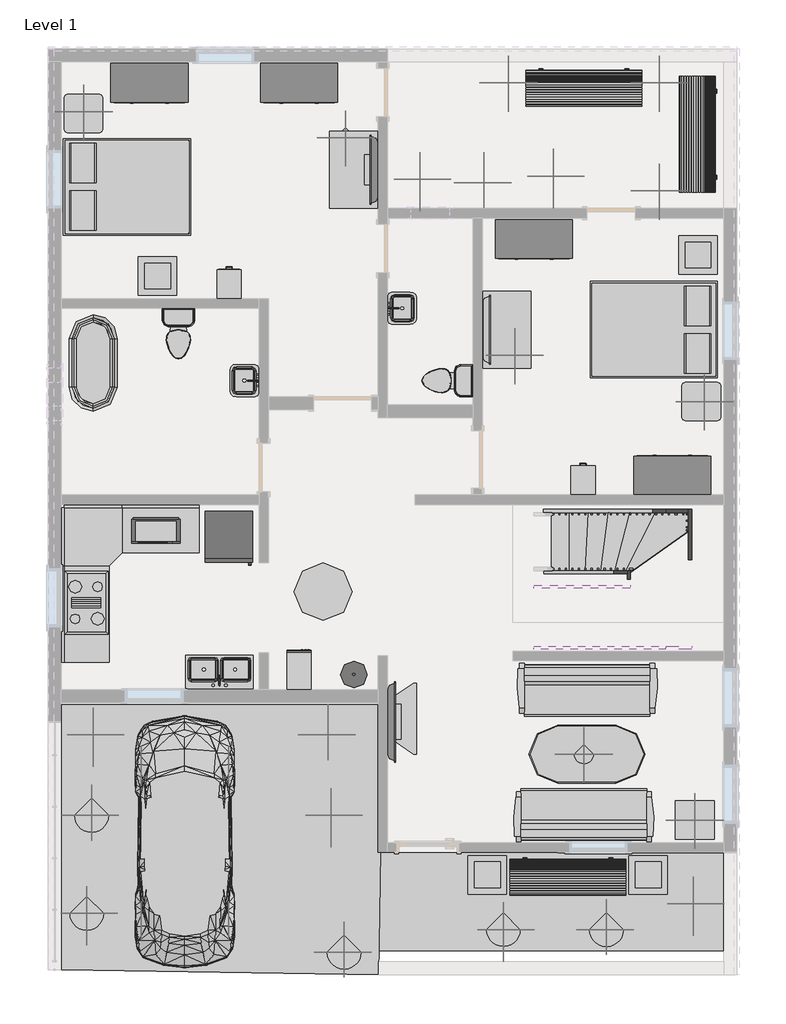
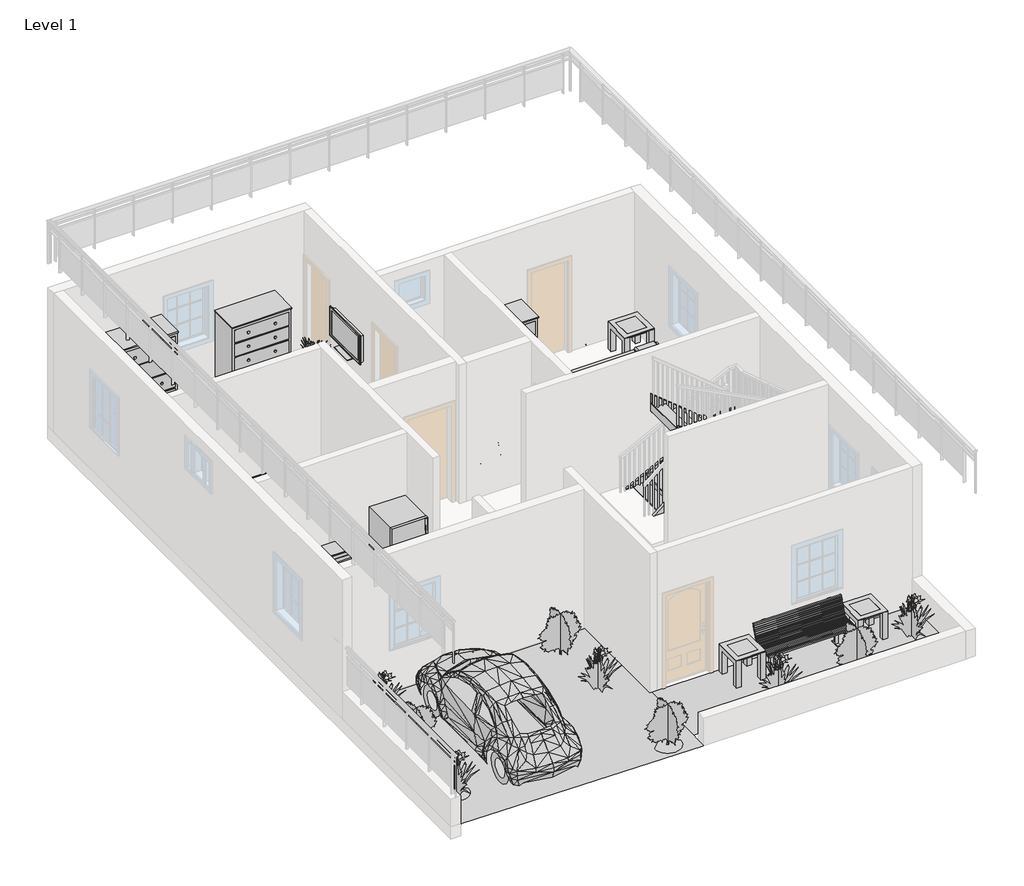
# One storey, part 4 of 4: 26 furniture elements, 24 geographic elements, 9 flow terminals, 8 members, 8 proxies, 1 stair flight.
"""IFC4 building model written with IfcOpenShell, lengths in millimetres."""

from ifc_helpers import new_model, si_unit, frame, origin, place, context, project, spatial, polyline, outline, extrude, triangles, transform, mapped, element, save
from components import proxy_db4bb64d, proxy_bb1e6e30, proxy_8a8d5ab2, rpc_beetle_rpc_beetle_3ce7ba48, proxy_a13a33b2, flow_terminal_2b63360b, flow_terminal_a53be723, flow_terminal_d49f872f, flow_terminal_62a433f7, toilet_domestic_3d_toilet_domestic_3d_f7549cf7, toilet_domestic_3d_toilet_domestic_3d_183bbd19, flow_terminal_b374fae2, furniture_1d2926bd, furniture_bb55ed6b, furniture_2babcf72, furniture_9fa109b2, furniture_aff9b2fb, furniture_7a3aaa4f, furniture_fdf74506, tv_stand_tv_stand_6ce107e5, furniture_b5c51a22, furniture_2c34a4f9, furniture_905aceb5, furniture_31d08a24, furniture_5bc9ed15, furniture_1bba2e14, furniture_3226db35, geographic_element_235d1464, rpc_plant_tropical_55f6ff97, rpc_plant_tropical_agave_1_5_93a2a214, rpc_plant_tropical_jungle_flame_3_9c4808c2, stair_flight_bfa9ce03

model = new_model("IFC4")

# Units and contexts
model_context = context("Model", 3, world=origin())
ifc_project = project(units=[si_unit("LENGTHUNIT", "METRE", prefix="MILLI")], contexts=[model_context])

# Site, building, storey
site = spatial("IfcSite", under=ifc_project)
building = spatial("IfcBuilding", under=site)
storey = spatial("IfcBuildingStorey", under=building, Name="Level 1", Elevation=0.0)

# Proxies
placement = place(None, origin())
element("IfcBuildingElementProxy", 1, Name="Building Element Proxy", at=placement, inside=storey, context=model_context, shape_type="Tessellation", body=[
    triangles([(-7623.7869781, 15698.6789795, 0.0), (-7623.7869781, 13031.6789795, 0.0), (-2111.986639, 15698.6789795, 0.0), (-2111.986639, 13184.0789795, 0.0)], [[1, 2, 4], [4, 3, 1]], closed=False),
])
element("IfcBuildingElementProxy", 2, Name="Building Element Proxy", at=placement, inside=storey, context=model_context, shape_type="Tessellation", body=[
    triangles([(-12983.1865906, 5475.1785919, 0.0), (-7699.9869781, 5487.8789795, 0.0), (-7763.4865906, 1474.6787373, 0.0), (-12983.1865906, 1576.2787857, 0.0), (-12779.986203, 1169.8788099, 0.0), (-7763.4865906, 1093.6788099, 0.0)], [[2, 1, 4], [3, 4, 5], [3, 6, 2], [6, 3, 5], [3, 2, 4]], closed=False),
])
element("IfcBuildingElementProxy", 3, Name="Building Element Proxy", at=placement, inside=storey, context=model_context, shape_type="Tessellation", body=[
    triangles([(-7776.1869781, 3024.0787857, 0.0), (-7763.4865906, 1474.6787373, 0.0), (-2111.986639, 3011.3786888, 0.0), (-2111.986639, 1474.6787373, 0.0)], [[1, 2, 3], [4, 3, 2]], closed=False),
])
proxy_shape = proxy_db4bb64d(model_context)
element("IfcBuildingElementProxy", 4, Name="15\" x 24\" x 34 1/2\"", ObjectType="15\" x 24\" x 34 1/2\"", at=placement, inside=storey, context=model_context, shape_type="MappedRepresentation", body=[
    mapped(proxy_shape, transform((-8752.769227, 6160.7283581, 0.0), x_axis=(-0.9999999999999998, 0.0, 0.0), y_axis=(0.0, -0.9999999999999998, 0.0), z_axis=(0.0, 0.0, 1.0))),
])
proxy_2_shape = proxy_bb1e6e30(model_context)
element("IfcBuildingElementProxy", 5, Name="Cook Top-4 Unit : 36\" x 20\"", ObjectType="Cook Top-4 Unit : 36\" x 20\"", at=placement, inside=storey, context=model_context, shape_type="MappedRepresentation", body=[
    mapped(proxy_2_shape, transform((-12379.9366955, 6961.0787933, 0.0), x_axis=(0.0, 1.0000000000000002, 0.0), y_axis=(-1.0000000000000002, 0.0, 0.0), z_axis=(0.0, 0.0, 1.0))),
])
proxy_3_shape = proxy_8a8d5ab2(model_context)
element("IfcBuildingElementProxy", 6, Name="Microwave : 30\" x 16\" x 18\"", ObjectType="Microwave : 30\" x 16\" x 18\"", at=placement, inside=storey, context=model_context, shape_type="MappedRepresentation", body=[
    mapped(proxy_3_shape, transform((-11781.6795729, 8457.1592991, 0.0), x_axis=(1.0000000000000009, 0.0, 0.0), y_axis=(0.0, 1.0000000000000009, 0.0), z_axis=(0.0, 0.0, 1.0))),
])
rpc_beetle_rpc_beetle_shape = rpc_beetle_rpc_beetle_3ce7ba48(model_context)
element("IfcBuildingElementProxy", 7, Name="RPC Beetle : RPC Beetle", ObjectType="RPC Beetle : RPC Beetle", at=placement, inside=storey, context=model_context, shape_type="MappedRepresentation", body=[
    mapped(rpc_beetle_rpc_beetle_shape, transform((-10824.1866955, 1957.2787933, 0.0), x_axis=(1.0, 0.0, 0.0), y_axis=(0.0, 1.0, 0.0), z_axis=(0.0, 0.0, 1.0))),
])
proxy_4_shape = proxy_a13a33b2(model_context)
element("IfcBuildingElementProxy", 8, Name="Refrigerator : 30\" x 32\" RH", ObjectType="Refrigerator : 30\" x 32\" RH", at=placement, inside=storey, context=model_context, shape_type="MappedRepresentation", body=[
    mapped(proxy_4_shape, transform((-10130.4491955, 8020.3298218, 0.0), x_axis=(1.0, 0.0, 0.0), y_axis=(0.0, 1.0, 0.0), z_axis=(0.0, 0.0, 1.0))),
])

# Flow terminals
flow_terminal_shape = flow_terminal_2b63360b(model_context)
element("IfcFlowTerminal", 9, ObjectType="Floor Drain - Rectangular : 5\"x5\" Strainer - 2\" Drain", at=placement, inside=storey, context=model_context, shape_type="MappedRepresentation", body=[
    mapped(flow_terminal_shape, transform((-11687.7866955, 11152.0787933, 0.0), x_axis=(1.0, 0.0, 0.0), y_axis=(0.0, 1.0, 0.0), z_axis=(0.0, 0.0, 1.0))),
])
element("IfcFlowTerminal", 10, ObjectType="Floor Drain - Rectangular : 5\"x5\" Strainer - 2\" Drain", at=placement, inside=storey, context=model_context, shape_type="MappedRepresentation", body=[
    mapped(flow_terminal_shape, transform((-7420.5866955, 10694.8787933, 0.0), x_axis=(1.0, 0.0, 0.0), y_axis=(0.0, 1.0, 0.0), z_axis=(0.0, 0.0, 1.0))),
])
flow_terminal_2_shape = flow_terminal_a53be723(model_context)
element("IfcFlowTerminal", 11, ObjectType="Sink Kitchen-Double : 42\" x 21\"", at=placement, inside=storey, context=model_context, shape_type="MappedRepresentation", body=[
    mapped(flow_terminal_2_shape, transform((-10262.397455, 5871.2241944, 0.0), x_axis=(-1.0000000000000004, 0.0, 0.0), y_axis=(0.0, -1.0000000000000004, 0.0), z_axis=(0.0, 0.0, 1.0))),
])
flow_terminal_3_shape = flow_terminal_d49f872f(model_context)
element("IfcFlowTerminal", 12, ObjectType="Sink Vanity-Round : 19\" x 19\"", at=placement, inside=storey, context=model_context, shape_type="MappedRepresentation", body=[
    mapped(flow_terminal_3_shape, transform((-8060.534955, 5914.6658677, 609.6), x_axis=(-1.0000000000000004, 0.0, 0.0), y_axis=(0.0, -1.0000000000000004, 0.0), z_axis=(0.0, 0.0, 1.0))),
])
flow_terminal_4_shape = flow_terminal_62a433f7(model_context)
element("IfcFlowTerminal", 13, ObjectType="Sink Vanity-Square : 20\" x 18\"", at=placement, inside=storey, context=model_context, shape_type="MappedRepresentation", body=[
    mapped(flow_terminal_4_shape, transform((-9835.9320966, 10481.9680338, 0.0), x_axis=(0.0, -0.9999999999999999, 0.0), y_axis=(0.9999999999999999, 0.0, 0.0), z_axis=(0.0, 0.0, 1.0))),
])
element("IfcFlowTerminal", 14, ObjectType="Sink Vanity-Square : 20\" x 18\"", at=placement, inside=storey, context=model_context, shape_type="MappedRepresentation", body=[
    mapped(flow_terminal_4_shape, transform((-7443.6412944, 11593.5895527, 0.0), x_axis=(0.0, 1.0000000000000002, 0.0), y_axis=(-1.0000000000000002, 0.0, 0.0), z_axis=(0.0, 0.0, 1.0))),
])
toilet_domestic_3d_toilet_domestic_3d_shape = toilet_domestic_3d_toilet_domestic_3d_f7549cf7(model_context)
toilet_domestic_3d_toilet_domestic_3d_2_shape = toilet_domestic_3d_toilet_domestic_3d_183bbd19(model_context)
element("IfcFlowTerminal", 15, ObjectType="Toilet-Domestic-3D : Toilet-Domestic-3D", at=placement, inside=storey, context=model_context, shape_type="MappedRepresentation", body=[
    mapped(toilet_domestic_3d_toilet_domestic_3d_shape, transform((-10925.7866955, 11114.5827659, 0.0), x_axis=(1.0, 0.0, 0.0), y_axis=(0.0, 1.0, 0.0), z_axis=(0.0, 0.0, 1.0))),
    mapped(toilet_domestic_3d_toilet_domestic_3d_2_shape, transform((-10925.7866955, 11114.5827659, 0.0), x_axis=(1.0, 0.0, 0.0), y_axis=(0.0, 1.0, 0.0), z_axis=(0.0, 0.0, 1.0))),
])
element("IfcFlowTerminal", 16, ObjectType="Toilet-Domestic-3D : Toilet-Domestic-3D", at=placement, inside=storey, context=model_context, shape_type="MappedRepresentation", body=[
    mapped(toilet_domestic_3d_toilet_domestic_3d_shape, transform((-6772.2827229, 10466.2787933, 0.0), x_axis=(0.0, -1.0, 0.0), y_axis=(1.0, 0.0, 0.0), z_axis=(0.0, 0.0, 1.0))),
    mapped(toilet_domestic_3d_toilet_domestic_3d_2_shape, transform((-6772.2827229, 10466.2787933, 0.0), x_axis=(0.0, -1.0, 0.0), y_axis=(1.0, 0.0, 0.0), z_axis=(0.0, 0.0, 1.0))),
])
flow_terminal_5_shape = flow_terminal_b374fae2(model_context)
element("IfcFlowTerminal", 17, ObjectType="Tub-Free Standing-3D : 30\" x 60\"", at=placement, inside=storey, context=model_context, shape_type="MappedRepresentation", body=[
    mapped(flow_terminal_5_shape, transform((-12271.9866955, 10745.6787933, 0.0), x_axis=(1.0, 0.0, 0.0), y_axis=(0.0, 1.0, 0.0), z_axis=(0.0, 0.0, 1.0))),
])

# Furniture
furniture_shape = furniture_1d2926bd(model_context)
element("IfcFurniture", 18, ObjectType="Bed-Box : Queen 60\" x 79\"", at=placement, inside=storey, context=model_context, shape_type="MappedRepresentation", body=[
    mapped(furniture_shape, transform((-11973.0162037, 13184.0787933, 0.0), x_axis=(0.0, 1.0000000000000002, 0.0), y_axis=(-1.0000000000000002, 0.0, 0.0), z_axis=(0.0, 0.0, 1.0))),
])
element("IfcFurniture", 19, ObjectType="Bed-Box : Queen 60\" x 79\"", at=placement, inside=storey, context=model_context, shape_type="MappedRepresentation", body=[
    mapped(furniture_shape, transform((-3185.6571873, 11609.2787933, 0.0), x_axis=(0.0, -1.0000000000000009, 0.0), y_axis=(1.0000000000000009, 0.0, 0.0), z_axis=(0.0, 0.0, 1.0))),
])
furniture_2_shape = furniture_bb55ed6b(model_context)
element("IfcFurniture", 20, ObjectType="Cabinet-File 2 Drawer : 15\" x 18\"", at=placement, inside=storey, context=model_context, shape_type="MappedRepresentation", body=[
    mapped(furniture_2_shape, transform((-10253.5831426, 11848.1444931, 0.0), x_axis=(-1.0000000000000002, 0.0, 0.0), y_axis=(0.0, -1.0000000000000002, 0.0), z_axis=(0.0, 0.0, 1.0))),
])
element("IfcFurniture", 21, ObjectType="Cabinet-File 2 Drawer : 15\" x 18\"", at=placement, inside=storey, context=model_context, shape_type="MappedRepresentation", body=[
    mapped(furniture_2_shape, transform((-4665.5831426, 8749.3444931, 0.0), x_axis=(-1.0, 0.0, 0.0), y_axis=(0.0, -1.0, 0.0), z_axis=(0.0, 0.0, 1.0))),
])
furniture_3_shape = furniture_2babcf72(model_context)
element("IfcFurniture", 22, ObjectType="Dresser : 48\" x 60\" x 24\"", at=placement, inside=storey, context=model_context, shape_type="MappedRepresentation", body=[
    mapped(furniture_3_shape, transform((-8751.5934357, 15528.4417474, 0.0), x_axis=(1.0, 0.0, 0.0), y_axis=(0.0, 1.0, 0.0), z_axis=(0.0, 0.0, 1.0))),
])
element("IfcFurniture", 23, ObjectType="Dresser : 48\" x 60\" x 24\"", at=placement, inside=storey, context=model_context, shape_type="MappedRepresentation", body=[
    mapped(furniture_3_shape, transform((-5043.1934357, 13064.6417474, 0.0), x_axis=(1.0, 0.0, 0.0), y_axis=(0.0, 1.0, 0.0), z_axis=(0.0, 0.0, 1.0))),
])
furniture_4_shape = furniture_9fa109b2(model_context)
element("IfcFurniture", 24, ObjectType="Dresser : 48\" x 72\" x 24\"", at=placement, inside=storey, context=model_context, shape_type="MappedRepresentation", body=[
    mapped(furniture_4_shape, transform((-11113.7934357, 15528.4417474, 0.0), x_axis=(1.0, 0.0, 0.0), y_axis=(0.0, 1.0, 0.0), z_axis=(0.0, 0.0, 1.0))),
])
element("IfcFurniture", 25, ObjectType="Dresser : 48\" x 72\" x 24\"", at=placement, inside=storey, context=model_context, shape_type="MappedRepresentation", body=[
    mapped(furniture_4_shape, transform((-3397.1799554, 8604.5158392, 0.0), x_axis=(-1.000000000000001, 0.0, 0.0), y_axis=(0.0, -1.000000000000001, 0.0), z_axis=(0.0, 0.0, 1.0))),
])
furniture_5_shape = furniture_aff9b2fb(model_context)
element("IfcFurniture", 26, ObjectType="Sofa-Pensi : 84\"", at=placement, inside=storey, context=model_context, shape_type="MappedRepresentation", body=[
    mapped(furniture_5_shape, transform((-4246.3804455, 3885.3886293, 0.0), x_axis=(-1.0000000000000004, 0.0, 0.0), y_axis=(0.0, -1.0000000000000004, 0.0), z_axis=(0.0, 0.0, 1.0))),
])
element("IfcFurniture", 27, ObjectType="Sofa-Pensi : 84\"", at=placement, inside=storey, context=model_context, shape_type="MappedRepresentation", body=[
    mapped(furniture_5_shape, transform((-4752.7929455, 5312.3689572, 0.0), x_axis=(1.0000000000000002, 0.0, 0.0), y_axis=(0.0, 1.0000000000000002, 0.0), z_axis=(0.0, 0.0, 1.0))),
])
furniture_6_shape = furniture_7a3aaa4f(model_context)
element("IfcFurniture", 28, ObjectType="TV - Flat Screen : 42\"", at=placement, inside=storey, context=model_context, shape_type="MappedRepresentation", body=[
    mapped(furniture_6_shape, transform((-7834.7253192, 13789.7342791, 990.6), x_axis=(0.0, -1.0000000000000004, 0.0), y_axis=(1.0000000000000004, 0.0, 0.0), z_axis=(0.0, 0.0, 1.0))),
])
element("IfcFurniture", 29, ObjectType="TV - Flat Screen : 42\"", at=placement, inside=storey, context=model_context, shape_type="MappedRepresentation", body=[
    mapped(furniture_6_shape, transform((-6066.6480719, 11274.0708484, 0.0), x_axis=(0.0, 1.0000000000000002, 0.0), y_axis=(-1.0000000000000002, 0.0, 0.0), z_axis=(0.0, 0.0, 1.0))),
])
furniture_7_shape = furniture_fdf74506(model_context)
element("IfcFurniture", 30, ObjectType="TV - Flat Screen : 50\"", at=placement, inside=storey, context=model_context, shape_type="MappedRepresentation", body=[
    mapped(furniture_7_shape, transform((-7565.2480719, 5085.4233074, 914.4), x_axis=(0.0, 1.0000000000000002, 0.0), y_axis=(-1.0000000000000002, 0.0, 0.0), z_axis=(0.0, 0.0, 1.0))),
])
tv_stand_tv_stand_shape = tv_stand_tv_stand_6ce107e5(model_context)
element("IfcFurniture", 31, ObjectType="TV Stand : TV Stand", at=placement, inside=storey, context=model_context, shape_type="MappedRepresentation", body=[
    mapped(tv_stand_tv_stand_shape, transform((-7623.7866955, 5007.0907912, 0.0), x_axis=(0.0, 1.0000000000000002, 0.0), y_axis=(-1.0000000000000002, 0.0, 0.0), z_axis=(0.0, 0.0, 1.0))),
])
furniture_8_shape = furniture_b5c51a22(model_context)
element("IfcFurniture", 32, ObjectType="Table-Coffee : 24\" x 24\" x 24\"", at=placement, inside=storey, context=model_context, shape_type="MappedRepresentation", body=[
    mapped(furniture_8_shape, transform((-11274.2524622, 12022.0677155, 0.0), x_axis=(1.0, 0.0, 0.0), y_axis=(0.0, 1.0, 0.0), z_axis=(0.0, 0.0, 1.0))),
])
element("IfcFurniture", 33, ObjectType="Table-Coffee : 24\" x 24\" x 24\"", at=placement, inside=storey, context=model_context, shape_type="MappedRepresentation", body=[
    mapped(furniture_8_shape, transform((-2739.8524622, 12352.2677155, 0.0), x_axis=(1.0, 0.0, 0.0), y_axis=(0.0, 1.0, 0.0), z_axis=(0.0, 0.0, 1.0))),
])
element("IfcFurniture", 34, ObjectType="Table-Coffee : 24\" x 24\" x 24\"", at=placement, inside=storey, context=model_context, shape_type="MappedRepresentation", body=[
    mapped(furniture_8_shape, transform((-6067.2524622, 2573.2677155, 0.0), x_axis=(1.0, 0.0, 0.0), y_axis=(0.0, 1.0, 0.0), z_axis=(0.0, 0.0, 1.0))),
])
element("IfcFurniture", 35, ObjectType="Table-Coffee : 24\" x 24\" x 24\"", at=placement, inside=storey, context=model_context, shape_type="MappedRepresentation", body=[
    mapped(furniture_8_shape, transform((-3527.2524622, 2573.2677155, 0.0), x_axis=(1.0, 0.0, 0.0), y_axis=(0.0, 1.0, 0.0), z_axis=(0.0, 0.0, 1.0))),
])
furniture_9_shape = furniture_2c34a4f9(model_context)
element("IfcFurniture", 36, ObjectType="Table-Dining Oval : 36\" x 72\"", at=placement, inside=storey, context=model_context, shape_type="MappedRepresentation", body=[
    mapped(furniture_9_shape, transform((-4072.3670234, 4931.5771539, 0.0), x_axis=(1.0, 0.0, 0.0), y_axis=(0.0, 1.0, 0.0), z_axis=(0.0, 0.0, 1.0))),
])
furniture_10_shape = furniture_905aceb5(model_context)
element("IfcFurniture", 37, ObjectType="Table-Dining Round w Chairs : 36\" Diameter", at=placement, inside=storey, context=model_context, shape_type="MappedRepresentation", body=[
    mapped(furniture_10_shape, transform((-8743.4686627, 7323.7574818, 0.0), x_axis=(1.0, 0.0, 0.0), y_axis=(0.0, 1.0, 0.0), z_axis=(0.0, 0.0, 1.0))),
])
furniture_11_shape = furniture_31d08a24(model_context)
element("IfcFurniture", 38, ObjectType="Table-End : 24\" x 24\"", at=placement, inside=storey, context=model_context, shape_type="MappedRepresentation", body=[
    mapped(furniture_11_shape, transform((-12732.9203258, 14530.2787933, 0.0), x_axis=(1.0, 0.0, 0.0), y_axis=(0.0, 1.0, 0.0), z_axis=(0.0, 0.0, 1.0))),
])
element("IfcFurniture", 39, ObjectType="Table-End : 24\" x 24\"", at=placement, inside=storey, context=model_context, shape_type="MappedRepresentation", body=[
    mapped(furniture_11_shape, transform((-2979.3203258, 9983.6787933, 0.0), x_axis=(1.0, 0.0, 0.0), y_axis=(0.0, 1.0, 0.0), z_axis=(0.0, 0.0, 1.0))),
])
furniture_12_shape = furniture_5bc9ed15(model_context)
element("IfcFurniture", 40, ObjectType="Table-Night Stand : 24\" x 24\" x 30\"", at=placement, inside=storey, context=model_context, shape_type="MappedRepresentation", body=[
    mapped(furniture_12_shape, transform((-2463.8530652, 3836.8787933, 0.0), x_axis=(-1.0000000000000004, 0.0, 0.0), y_axis=(0.0, -1.0000000000000004, 0.0), z_axis=(0.0, 0.0, 1.0))),
])
furniture_13_shape = furniture_1bba2e14(model_context)
element("IfcFurniture", 41, ObjectType="Table-Rectangular : 72\" x 30\"", at=placement, inside=storey, context=model_context, shape_type="MappedRepresentation", body=[
    mapped(furniture_13_shape, transform((-8157.1866955, 13793.6787933, 0.0), x_axis=(0.0, 1.0000000000000002, 0.0), y_axis=(-1.0000000000000002, 0.0, 0.0), z_axis=(0.0, 0.0, 1.0))),
])
element("IfcFurniture", 42, ObjectType="Table-Rectangular : 72\" x 30\"", at=placement, inside=storey, context=model_context, shape_type="MappedRepresentation", body=[
    mapped(furniture_13_shape, transform((-5744.1866955, 11270.1263343, 0.0), x_axis=(0.0, 1.0000000000000002, 0.0), y_axis=(-1.0000000000000002, 0.0, 0.0), z_axis=(0.0, 0.0, 1.0))),
])
furniture_14_shape = furniture_3226db35(model_context)
element("IfcFurniture", 43, ObjectType="Work Station Cubicle : 96\" x 96\"", at=placement, inside=storey, context=model_context, shape_type="MappedRepresentation", body=[
    mapped(furniture_14_shape, transform((-12648.2549433, 9005.5018009, 0.0), x_axis=(1.0, 0.0, 0.0), y_axis=(0.0, 1.0, 0.0), z_axis=(0.0, 0.0, 1.0))),
])

# Geographic elements
geographic_element_shape = geographic_element_235d1464(model_context)
element("IfcGeographicElement", 44, ObjectType="Park Bench : 72\"", at=placement, inside=storey, context=model_context, shape_type="MappedRepresentation", body=[
    mapped(geographic_element_shape, transform((-4524.9866955, 15114.4787933, 0.0), x_axis=(1.0, 0.0, 0.0), y_axis=(0.0, 1.0, 0.0), z_axis=(0.0, 0.0, 1.0))),
])
element("IfcGeographicElement", 45, ObjectType="Park Bench : 72\"", at=placement, inside=storey, context=model_context, shape_type="MappedRepresentation", body=[
    mapped(geographic_element_shape, transform((-2696.1866955, 14352.4787933, 0.0), x_axis=(0.0, -1.0000000000000004, 0.0), y_axis=(1.0000000000000004, 0.0, 0.0), z_axis=(0.0, 0.0, 1.0))),
])
element("IfcGeographicElement", 46, ObjectType="Park Bench : 72\"", at=placement, inside=storey, context=model_context, shape_type="MappedRepresentation", body=[
    mapped(geographic_element_shape, transform((-4778.9866955, 2668.4787933, 0.0), x_axis=(1.0, 0.0, 0.0), y_axis=(0.0, 1.0, 0.0), z_axis=(0.0, 0.0, 1.0))),
])
rpc_plant_tropical_shape = rpc_plant_tropical_55f6ff97(model_context)
element("IfcGeographicElement", 47, ObjectType="RPC Plant - Tropical", at=placement, inside=storey, context=model_context, shape_type="MappedRepresentation", body=[
    mapped(rpc_plant_tropical_shape, transform((-7115.7866955, 13641.2787933, 0.0), x_axis=(1.0, 0.0, 0.0), y_axis=(0.0, 1.0, 0.0), z_axis=(0.0, 0.0, 1.0))),
])
element("IfcGeographicElement", 48, ObjectType="RPC Plant - Tropical", at=placement, inside=storey, context=model_context, shape_type="MappedRepresentation", body=[
    mapped(rpc_plant_tropical_shape, transform((-5007.5866955, 13692.0787933, 0.0), x_axis=(1.0, 0.0, 0.0), y_axis=(0.0, 1.0, 0.0), z_axis=(0.0, 0.0, 1.0))),
])
element("IfcGeographicElement", 49, ObjectType="RPC Plant - Tropical", at=placement, inside=storey, context=model_context, shape_type="MappedRepresentation", body=[
    mapped(rpc_plant_tropical_shape, transform((-12271.9866955, 4878.2787933, 0.0), x_axis=(1.0, 0.0, 0.0), y_axis=(0.0, 1.0, 0.0), z_axis=(0.0, 0.0, 1.0))),
])
element("IfcGeographicElement", 50, ObjectType="RPC Plant - Tropical", at=placement, inside=storey, context=model_context, shape_type="MappedRepresentation", body=[
    mapped(rpc_plant_tropical_shape, transform((-12373.5866955, 2058.8787933, 0.0), x_axis=(1.0, 0.0, 0.0), y_axis=(0.0, 1.0, 0.0), z_axis=(0.0, 0.0, 1.0))),
])
element("IfcGeographicElement", 51, ObjectType="RPC Plant - Tropical", at=placement, inside=storey, context=model_context, shape_type="MappedRepresentation", body=[
    mapped(rpc_plant_tropical_shape, transform((-8512.7866955, 3608.2787933, 0.0), x_axis=(1.0, 0.0, 0.0), y_axis=(0.0, 1.0, 0.0), z_axis=(0.0, 0.0, 1.0))),
])
element("IfcGeographicElement", 52, ObjectType="RPC Plant - Tropical", at=placement, inside=storey, context=model_context, shape_type="MappedRepresentation", body=[
    mapped(rpc_plant_tropical_shape, transform((-2797.7866955, 2211.2787933, 0.0), x_axis=(1.0, 0.0, 0.0), y_axis=(0.0, 1.0, 0.0), z_axis=(0.0, 0.0, 1.0))),
])
element("IfcGeographicElement", 53, ObjectType="RPC Plant - Tropical", at=placement, inside=storey, context=model_context, shape_type="MappedRepresentation", body=[
    mapped(rpc_plant_tropical_shape, transform((-5794.9866955, 1804.8787933, 0.0), x_axis=(1.0, 0.0, 0.0), y_axis=(0.0, 1.0, 0.0), z_axis=(0.0, 0.0, 1.0))),
])
rpc_plant_tropical_agave_1_5_shape = rpc_plant_tropical_agave_1_5_93a2a214(model_context)
element("IfcGeographicElement", 54, ObjectType="RPC Plant - Tropical : Agave - 1.5'", at=placement, inside=storey, context=model_context, shape_type="MappedRepresentation", body=[
    mapped(rpc_plant_tropical_agave_1_5_shape, transform((-12424.3866955, 14708.0787933, 609.6), x_axis=(1.0, 0.0, 0.0), y_axis=(0.0, 1.0, 0.0), z_axis=(0.0, 0.0, 1.0))),
])
element("IfcGeographicElement", 55, ObjectType="RPC Plant - Tropical : Agave - 1.5'", at=placement, inside=storey, context=model_context, shape_type="MappedRepresentation", body=[
    mapped(rpc_plant_tropical_agave_1_5_shape, transform((-8284.1866955, 14301.6787933, 609.6), x_axis=(1.0, 0.0, 0.0), y_axis=(0.0, 1.0, 0.0), z_axis=(0.0, 0.0, 1.0))),
])
element("IfcGeographicElement", 56, ObjectType="RPC Plant - Tropical : Agave - 1.5'", at=placement, inside=storey, context=model_context, shape_type="MappedRepresentation", body=[
    mapped(rpc_plant_tropical_agave_1_5_shape, transform((-3331.1866955, 15165.2787933, 0.0), x_axis=(1.0, 0.0, 0.0), y_axis=(0.0, 1.0, 0.0), z_axis=(0.0, 0.0, 1.0))),
])
element("IfcGeographicElement", 57, ObjectType="RPC Plant - Tropical : Agave - 1.5'", at=placement, inside=storey, context=model_context, shape_type="MappedRepresentation", body=[
    mapped(rpc_plant_tropical_agave_1_5_shape, transform((-5718.7866955, 15165.2787933, 0.0), x_axis=(1.0, 0.0, 0.0), y_axis=(0.0, 1.0, 0.0), z_axis=(0.0, 0.0, 1.0))),
])
element("IfcGeographicElement", 58, ObjectType="RPC Plant - Tropical : Agave - 1.5'", at=placement, inside=storey, context=model_context, shape_type="MappedRepresentation", body=[
    mapped(rpc_plant_tropical_agave_1_5_shape, transform((-3331.1866955, 13463.4787933, 0.0), x_axis=(1.0, 0.0, 0.0), y_axis=(0.0, 1.0, 0.0), z_axis=(0.0, 0.0, 1.0))),
])
element("IfcGeographicElement", 59, ObjectType="RPC Plant - Tropical : Agave - 1.5'", at=placement, inside=storey, context=model_context, shape_type="MappedRepresentation", body=[
    mapped(rpc_plant_tropical_agave_1_5_shape, transform((-2619.9866955, 10136.0787933, 609.6), x_axis=(1.0, 0.0, 0.0), y_axis=(0.0, 1.0, 0.0), z_axis=(0.0, 0.0, 1.0))),
])
element("IfcGeographicElement", 60, ObjectType="RPC Plant - Tropical : Agave - 1.5'", at=placement, inside=storey, context=model_context, shape_type="MappedRepresentation", body=[
    mapped(rpc_plant_tropical_agave_1_5_shape, transform((-5617.1866955, 10863.7263343, 609.6), x_axis=(1.0, 0.0, 0.0), y_axis=(0.0, 1.0, 0.0), z_axis=(0.0, 0.0, 1.0))),
])
element("IfcGeographicElement", 61, ObjectType="RPC Plant - Tropical : Agave - 1.5'", at=placement, inside=storey, context=model_context, shape_type="MappedRepresentation", body=[
    mapped(rpc_plant_tropical_agave_1_5_shape, transform((-4524.9866955, 4573.4787933, 914.4), x_axis=(1.0, 0.0, 0.0), y_axis=(0.0, 1.0, 0.0), z_axis=(0.0, 0.0, 1.0))),
])
element("IfcGeographicElement", 62, ObjectType="RPC Plant - Tropical : Agave - 1.5'", at=placement, inside=storey, context=model_context, shape_type="MappedRepresentation", body=[
    mapped(rpc_plant_tropical_agave_1_5_shape, transform((-2772.3866955, 3532.0787933, 762.0), x_axis=(1.0, 0.0, 0.0), y_axis=(0.0, 1.0, 0.0), z_axis=(0.0, 0.0, 1.0))),
])
rpc_plant_tropical_jungle_flame_3_shape = rpc_plant_tropical_jungle_flame_3_9c4808c2(model_context)
element("IfcGeographicElement", 63, ObjectType="RPC Plant - Tropical : Jungle Flame - 3'", at=placement, inside=storey, context=model_context, shape_type="MappedRepresentation", body=[
    mapped(rpc_plant_tropical_jungle_flame_3_shape, transform((-6099.7866955, 13590.4787933, 0.0), x_axis=(1.0, 0.0, 0.0), y_axis=(0.0, 1.0, 0.0), z_axis=(0.0, 0.0, 1.0))),
])
element("IfcGeographicElement", 64, ObjectType="RPC Plant - Tropical : Jungle Flame - 3'", at=placement, inside=storey, context=model_context, shape_type="MappedRepresentation", body=[
    mapped(rpc_plant_tropical_jungle_flame_3_shape, transform((-12297.3866955, 3608.2787933, 0.0), x_axis=(1.0, 0.0, 0.0), y_axis=(0.0, 1.0, 0.0), z_axis=(0.0, 0.0, 1.0))),
])
element("IfcGeographicElement", 65, ObjectType="RPC Plant - Tropical : Jungle Flame - 3'", at=placement, inside=storey, context=model_context, shape_type="MappedRepresentation", body=[
    mapped(rpc_plant_tropical_jungle_flame_3_shape, transform((-8563.5866955, 4878.2787933, 0.0), x_axis=(1.0, 0.0, 0.0), y_axis=(0.0, 1.0, 0.0), z_axis=(0.0, 0.0, 1.0))),
])
element("IfcGeographicElement", 66, ObjectType="RPC Plant - Tropical : Jungle Flame - 3'", at=placement, inside=storey, context=model_context, shape_type="MappedRepresentation", body=[
    mapped(rpc_plant_tropical_jungle_flame_3_shape, transform((-8309.5866955, 1449.2787933, 0.0), x_axis=(1.0, 0.0, 0.0), y_axis=(0.0, 1.0, 0.0), z_axis=(0.0, 0.0, 1.0))),
])
element("IfcGeographicElement", 67, ObjectType="RPC Plant - Tropical : Jungle Flame - 3'", at=placement, inside=storey, context=model_context, shape_type="MappedRepresentation", body=[
    mapped(rpc_plant_tropical_jungle_flame_3_shape, transform((-4169.3866955, 1804.8787933, 0.0), x_axis=(1.0, 0.0, 0.0), y_axis=(0.0, 1.0, 0.0), z_axis=(0.0, 0.0, 1.0))),
])

# Members
element("IfcMember", 68, ObjectType="Stringer - 2\" Width", at=placement, inside=storey, context=model_context, shape_type="SweptSolid", body=[
    extrude(outline(polyline([(229.639954, -5316.1183874), (0.0, -5316.1183874), (0.0, -5096.3560698), (962.500629, -3228.7011957), (1305.3956453, -3228.7011957), (229.639954, -5316.1183874)])), frame((0.0, 8383.4787933, 0.0), z_axis=(0.0, 1.0, 0.0), x_axis=(0.0, 0.0, 1.0)), (0.0, 0.0, 1.0), 50.8),
])
element("IfcMember", 69, ObjectType="Stringer - 2\" Width", at=placement, inside=storey, context=model_context, shape_type="SweptSolid", body=[
    extrude(outline(polyline([(-3228.7011957, 8383.4787933), (-3228.7011957, 8434.2787933), (-2873.9866955, 8434.2787933), (-2873.9866955, 8383.4787933), (-3228.7011957, 8383.4787933)])), frame((0.0, 0.0, 962.500629), z_axis=(0.0, 0.0, 1.0), x_axis=(1.0, 0.0, 0.0)), (0.0, 0.0, 1.0), 342.8950162),
])
element("IfcMember", 70, ObjectType="Stringer - 2\" Width", at=placement, inside=storey, context=model_context, shape_type="SweptSolid", body=[
    extrude(outline(polyline([(8434.2787933, 1289.0952212), (8434.2787933, 1000.5956453), (8264.7563103, 1000.5956453), (6275.2787933, 1638.9682298), (6275.2787933, 1969.9972697), (6312.2589106, 1969.9972697), (8434.2787933, 1289.0952212)])), frame((-2873.9866955, 0.0, 0.0), z_axis=(1.0, 0.0, 0.0), x_axis=(0.0, 1.0, 0.0)), (0.0, 0.0, 1.0), 50.8),
])
element("IfcMember", 71, ObjectType="Stringer - 2\" Width", at=placement, inside=storey, context=model_context, shape_type="SweptSolid", body=[
    extrude(outline(polyline([(-2823.1866955, 6275.2787933), (-2823.1866955, 6224.4787933), (-3228.7011957, 6224.4787933), (-3228.7011957, 6275.2787933), (-2823.1866955, 6275.2787933)])), frame((0.0, 0.0, 1649.8904473), z_axis=(0.0, 0.0, 1.0), x_axis=(1.0, 0.0, 0.0)), (0.0, 0.0, 1.0), 320.1068224),
])
element("IfcMember", 72, ObjectType="Stringer - 2\" Width", at=placement, inside=storey, context=model_context, shape_type="SweptSolid", body=[
    extrude(outline(polyline([(1649.8904473, -3228.7011957), (1969.9972697, -3228.7011957), (3045.7529609, -5316.1183874), (2725.6461385, -5316.1183874), (1649.8904473, -3228.7011957)])), frame((0.0, 6224.4787933, 0.0), z_axis=(0.0, 1.0, 0.0), x_axis=(0.0, 0.0, 1.0)), (0.0, 0.0, 1.0), 50.8),
])
element("IfcMember", 73, ObjectType="Stringer - 2\" Width", at=placement, inside=storey, context=model_context, shape_type="SweptSolid", body=[
    extrude(outline(polyline([(176.1764461, -5316.1183874), (0.0, -5316.1183874), (0.0, -5049.8567428), (987.1410923, -3839.1866955), (1380.418648, -3839.1866955), (176.1764461, -5316.1183874)])), frame((0.0, 7418.2787933, 0.0), z_axis=(0.0, 1.0, 0.0), x_axis=(0.0, 0.0, 1.0)), (0.0, 0.0, 1.0), 50.8),
])
element("IfcMember", 74, ObjectType="Stringer - 2\" Width", at=placement, inside=storey, context=model_context, shape_type="SweptSolid", body=[
    extrude(outline(polyline([(7469.0787933, 1573.2682978), (7469.0787933, 1028.5617647), (7434.836576, 1028.5617647), (7240.4787933, 1360.465107), (7240.4787933, 1926.1409689), (7262.4416758, 1926.1409689), (7469.0787933, 1573.2682978)])), frame((-3839.1866955, 0.0, 0.0), z_axis=(1.0, 0.0, 0.0), x_axis=(0.0, 1.0, 0.0)), (0.0, 0.0, 1.0), 50.8),
])
element("IfcMember", 75, ObjectType="Stringer - 2\" Width", at=placement, inside=storey, context=model_context, shape_type="SweptSolid", body=[
    extrude(outline(polyline([(1532.8634131, -3788.3866955), (1926.1409689, -3788.3866955), (3171.8038432, -5316.1183874), (2778.5262875, -5316.1183874), (1532.8634131, -3788.3866955)])), frame((0.0, 7189.6787933, 0.0), z_axis=(0.0, 1.0, 0.0), x_axis=(0.0, 0.0, 1.0)), (0.0, 0.0, 1.0), 50.8),
])

# Stair flight
stair_flight_shape = stair_flight_bfa9ce03(model_context)
element("IfcStairFlight", 76, ObjectType="2\" Tread 1\" Nosing 1/4\" Riser", at=placement, inside=storey, context=model_context, shape_type="MappedRepresentation", body=[
    mapped(stair_flight_shape, transform((0.0, 0.0, 0.0), x_axis=(1.0, 0.0, 0.0), y_axis=(0.0, 1.0, 0.0), z_axis=(0.0, 0.0, 1.0))),
])

save(model, "model.ifc")

# Revit data of these elements
# Type "15\" x 24\" x 34 1/2\""
#   Label = "T"
#   Assembly Code = "E1090400"
#   Depth = 2' - 0"
#   Height = 2' - 10 1/2"
#   Width = 1' - 3"
#   Panel Face Material = Plastic, Opaque Black
#   Trach Compact. Material = Steel, Paint Finish, Ivory, Matte
#   Default Elevation = 0
# Type "Cook Top-4 Unit : 36\" x 20\""
#   Assembly Code = "E1090400"
#   Depth = 2' - 0"
#   Width = 3' - 0"
#   Burner Material = Steel, Chrome Plated
#   Cooktop Material = Steel, Polished
#   Default Elevation = 0
# Type "Microwave : 30\" x 16\" x 18\""
#   Assembly Code = "E1090400"
#   Depth = 1' - 4"
#   Height = 1' - 6"
#   Width = 2' - 6"
#   Microwave Material = Laminate, Ivory, Matte
#   Default Elevation = 0
# Type "RPC Beetle : RPC Beetle"
#   built-in parameter 1005195 = "RPC-16-0U6E-L4EG-ENH1-J3KF-SVEL-0TX4-C0"
#   Height = 0
# Type "Refrigerator : 30\" x 32\" RH"
#   Label = "REF."
#   Assembly Code = "E1090400"
#   Depth = 2' - 7 3/4"
#   Handle = 2' - 3"
#   Height = 5' - 10"
#   Rear Clearance = 0' - 2"
#   Top Door Height = 1' - 8"
#   Width = 2' - 5 3/8"
#   Material = Steel, Paint Finish, Ivory, Glossy
#   Default Elevation = 0
# Type "Floor Drain - Rectangular : 5\"x5\" Strainer - 2\" Drain"
#   WFU = 2
#   Strainer Height = 0' - 3 1/4"
#   Half Strainer Length = 0' - 2 1/2"
#   Strainer Length = 0' - 5"
#   Radius 2 = 0' - 3.04167"
#   Radius 1 = 0' - 2.02083"
#   Radius 3 = 0' - 2 1/32"
#   Pipe Radius = 1"
#   Pipe Diameter = 2"
#   Height 2 = 0' - 0.725"
#   Height 1 = 0' - 1 13/16"
#   Body Radius = 0' - 4 1/16"
#   Body Height = 0' - 3 5/8"
#   Body Diameter = 0' - 8 1/8"
#   Drain Material = none
#   HWFU = 0
#   Default Elevation = 0
#   CWFU = 0
# Type "Sink Kitchen-Double : 42\" x 21\""
#   Assembly Code = "D2010410"
#   Counter Height = 3' - 0"
#   Depth = 1' - 9"
#   Width = 3' - 6"
#   Faucet Material = Steel, Polished
#   Sink Material = Steel, Polished
#   Default Elevation = 0
# Type "Sink Vanity-Round : 19\" x 19\""
#   Assembly Code = "D2010400"
#   Top Of Counter = 2' - 7"
#   Basin Material = Porcelain, Linen
#   Faucet Material = Steel, Polished
#   Default Elevation = 0
# Type "Sink Vanity-Square : 20\" x 18\""
#   Assembly Code = "D2010400"
#   Counter Height = 2' - 7"
#   Depth = 1' - 6"
#   Width = 1' - 8"
#   Basin Material = Porcelain, Linen
#   Faucet Material = Steel, Polished
#   Default Elevation = 0
# Type "Toilet-Domestic-3D : Toilet-Domestic-3D"
#   Assembly Code = "D2010110"
#   Toilet - Bowl/Basin Material = Porcelain, Linen
#   Toilet - Seat Material = Laminate, Linen, Matte
#   Default Elevation = 0
# Type "Tub-Free Standing-3D : 30\" x 60\""
#   Assembly Code = "D2010110"
#   Height = 1' - 6"
#   Length = 5' - 0"
#   Width = 2' - 6"
#   Tub Material = Porcelain, Ivory
#   Default Elevation = 0
# Type "Bed-Box : Queen 60\" x 79\""
#   Assembly Code = "E2020200"
#   Length = 6' - 7"
#   Width = 5' - 0"
#   Frame Material = Birch
#   Mattress Material = Sash
#   Default Elevation = 0
# Type "Cabinet-File 2 Drawer : 15\" x 18\""
#   Assembly Code = "E2020200"
#   Depth = 1' - 6"
#   Height = 2' - 5"
#   Width = 1' - 3"
#   Cabinet Material = Steel, Paint Finish, Ivory, Glossy
#   Handle Material = Steel, Chrome Plated
#   Default Elevation = 0
# Type "Dresser : 48\" x 60\" x 24\""
#   Assembly Code = "E2020200"
#   Depth = 2' - 0"
#   Height = 5' - 0"
#   Width = 4' - 0"
#   Dresser Material = Laminate - Ivory, Glossy
#   Drawer Material = Laminate, Ivory, Matte
#   Knob Material = Cherry
#   Default Elevation = 0
# Type "Dresser : 48\" x 72\" x 24\""
#   Assembly Code = "E2020200"
#   Depth = 2' - 0"
#   Height = 6' - 0"
#   Width = 4' - 0"
#   Dresser Material = Wood - Teak
#   Drawer Material = Wood - Teak
#   Knob Material = Cherry
#   Default Elevation = 0
# Type "Sofa-Pensi : 84\""
#   Assembly Code = "E2020200"
#   Length = 7' - 0"
#   Frame Material = Cherry
#   Seat Material = Linen, Beige
#   Feet Material = Steel, Chrome Plated
#   Default Elevation = 0
# Type "TV - Flat Screen : 42\""
#   SinAng = 0' - 0.0193"
#   L = 3' - 0.71517"
#   H = 1' - 8.65418"
#   Thickness = 0' - 4.33071"
#   Diagonal = 3' - 6.12598"
#   CosAng = 0' - 0.03431"
#   Stand [instance default] = yes
#   Default Elevation = 0
# Type "TV - Flat Screen : 50\""
#   SinAng = 0' - 0.0193"
#   L = 3' - 7.57782"
#   H = 2' - 0.51477"
#   Thickness = 0' - 4.33071"
#   Diagonal = 4' - 2"
#   CosAng = 0' - 0.03431"
#   Stand [instance default] = yes
#   Default Elevation = 0
# Type "TV Stand : TV Stand"
#   Depth = 1' - 6"
#   Width = 3' - 8"
#   Height = 1' - 7 1/2"
#   Finish = Melamine - Gray
#   Default Elevation = 0
# Type "Table-Coffee : 24\" x 24\" x 24\""
#   Assembly Code = "E2020200"
#   Height = 2' - 0"
#   Length = 2' - 0"
#   Width = 2' - 0"
#   Top Material = none
#   Frame Material = none
#   Default Elevation = 0
# Type "Table-Dining Oval : 36\" x 72\""
#   Assembly Code = "E2020200"
#   Length = 6' - 0"
#   Width = 3' - 0"
#   Base Material = Steel, Chrome Plated
#   Top Material = Glass - Clear, Grey
#   Default Elevation = 0
#   Description = (empty or 0)
# Type "Table-Dining Round w Chairs : 36\" Diameter"
#   Assembly Code = "E2020200"
#   Radius = 1' - 6"
#   Diameter = 3' - 0"
#   Height = 2' - 6"
#   Chairs = 4
#   Base Material = Pine
#   Top Material = Laminate, Linen, Matte
#   Default Elevation = 0
# Type "Table-End : 24\" x 24\""
#   Assembly Code = "E2020200"
#   Height = 2' - 0"
#   Length = 2' - 0"
#   Width = 2' - 0"
#   Base Material = Birch
#   Top Material = Laminate, Ivory, Matte
#   Default Elevation = 0
# Type "Table-Night Stand : 24\" x 24\" x 30\""
#   Assembly Code = "E2020200"
#   Depth = 2' - 0"
#   Height = 2' - 6"
#   Width = 2' - 0"
#   Base Material = Birch
#   Top Material = Laminate, Ivory, Matte
#   Default Elevation = 0
# Type "Table-Rectangular : 72\" x 30\""
#   Assembly Code = "E2020200"
#   Height = 2' - 0"
#   Length = 4' - 0"
#   Width = 2' - 6"
#   Base Material = Birch
#   Top Material = Birch
#   Default Elevation = 0
# Type "Work Station Cubicle : 96\" x 96\""
#   Assembly Code = "E2020"
#   Desktop Height = 2' - 6"
#   Desktop1 Width = 2' - 4"
#   Desktop2 Width = 2' - 4"
#   Panel Height = 2' - 8"
#   Panel1 Length = 5' - 0"
#   Panel2 Length = 4' - 0"
#   Cube Panel Material = Textile - Light Gray
#   Work Top Material = Laminate, Ivory, Matte
#   Default Elevation = 0
# Type "Park Bench : 72\""
#   Length = 6' - 0"
#   Seat Material = Wood - Teak
#   Frame Material = Steel, Paint Finish, Dark Gray, Matte
# Type "RPC Plant - Tropical"
#   built-in parameter 1005198 = "{2, 15},{39, RPC-16-FWM5-GM7X-C67P-4000-ST1L-LVER-AU},{1, 0},{1, 0},{2, 13},{1, 8},{5, Color},{1, 0},{1, 0},{3, 0.8},{3, 0.8},{3, 0.8},{1, 8},{7, BBoxMin},{1, 0},{1, 0},{1, 0},{1, 0},{1, 0},{1, 8},{7, BBoxMax},{1, 0},{1, 0},{1, 0},{1, 0},{1, 0},{2, 11},{9, RPCTypeId},{1, 0},{1, 0},{39, RPC-16-FWM5-GM7X-C67P-4000-ST1L-LVER-AU},{1, 6},{14, RPCPlantHeight},{1, 0},{1, 0},{1, 3},{2, 11},{7, keyword},{1, 0},{1, 0},{35, :RPCs:Shrubs [General]:Geometry:RPC},{2, 11},{8, category},{1, 0},{1, 0},{16, Shrubs [General]},{2, 11},{12, LocalizedUID},{1, 0},{1, 0},{10, Crane Lily},{2, 14},{6, Height},{1, 0},{1, 0},{1, 3},{1, 2},{16, Cast Reflections},{1, 0},{1, 0},{1, 0},{1, 2},{12, Cast Shadows},{1, 0},{1, 0},{1, 1},{1, 2},{9, Lock View},{1, 0},{1, 0},{1, 0},{1, 4},{5, ViewC},{1, 0},{1, 0},{1, 0},{21, assetlibrary_base.fbx},{1, 5},"
#   built-in parameter 1005195 = "RPC-16-FWM5-GM7X-C67P-4000-ST1L-LVER-AU"
#   Assembly Code = "G2050500"
#   Height = 3' - 0"
#   Default Elevation = 0
# Type "RPC Plant - Tropical : Agave - 1.5'"
#   built-in parameter 1005198 = "{2, 15},{39, RPC-16-G1GJ-63FX-7K5P-N000-ST1L-LVER-AU},{1, 0},{1, 0},{2, 13},{1, 8},{5, Color},{1, 0},{1, 0},{3, 0.8},{3, 0.8},{3, 0.8},{1, 8},{7, BBoxMin},{1, 0},{1, 0},{1, 0},{1, 0},{1, 0},{1, 8},{7, BBoxMax},{1, 0},{1, 0},{1, 0},{1, 0},{1, 0},{2, 11},{9, RPCTypeId},{1, 0},{1, 0},{39, RPC-16-G1GJ-63FX-7K5P-N000-ST1L-LVER-AU},{1, 6},{14, RPCPlantHeight},{1, 0},{1, 0},{3, 1.5},{2, 11},{7, keyword},{1, 0},{1, 0},{35, :RPCs:Plants [General]:Geometry:RPC},{2, 11},{8, category},{1, 0},{1, 0},{16, Plants [General]},{2, 11},{12, LocalizedUID},{1, 0},{1, 0},{5, Agave},{2, 14},{6, Height},{1, 0},{1, 0},{3, 1.5},{1, 2},{16, Cast Reflections},{1, 0},{1, 0},{1, 0},{1, 2},{12, Cast Shadows},{1, 0},{1, 0},{1, 1},{1, 2},{9, Lock View},{1, 0},{1, 0},{1, 0},{1, 4},{5, ViewC},{1, 0},{1, 0},{1, 0},{21, assetlibrary_base.fbx},{1, 5},"
#   built-in parameter 1005195 = "RPC-16-G1GJ-63FX-7K5P-N000-ST1L-LVER-AU"
#   Type Comments = "Agave"
#   Assembly Code = "G2050500"
#   Height = 1' - 6"
#   Default Elevation = 0
# Type "RPC Plant - Tropical : Jungle Flame - 3'"
#   built-in parameter 1005198 = "{2, 15},{39, RPC-16-FUVJ-JWG0-MWGK-8000-ST1L-LVER-AU},{1, 0},{1, 0},{2, 13},{1, 8},{5, Color},{1, 0},{1, 0},{3, 0.8},{3, 0.8},{3, 0.8},{1, 8},{7, BBoxMin},{1, 0},{1, 0},{1, 0},{1, 0},{1, 0},{1, 8},{7, BBoxMax},{1, 0},{1, 0},{1, 0},{1, 0},{1, 0},{2, 11},{9, RPCTypeId},{1, 0},{1, 0},{39, RPC-16-FUVJ-JWG0-MWGK-8000-ST1L-LVER-AU},{1, 6},{14, RPCPlantHeight},{1, 0},{1, 0},{1, 3},{2, 11},{7, keyword},{1, 0},{1, 0},{35, :RPCs:Shrubs [General]:Geometry:RPC},{2, 11},{8, category},{1, 0},{1, 0},{16, Shrubs [General]},{2, 11},{12, LocalizedUID},{1, 0},{1, 0},{12, Jungle Flame},{2, 14},{6, Height},{1, 0},{1, 0},{1, 3},{1, 2},{16, Cast Reflections},{1, 0},{1, 0},{1, 0},{1, 2},{12, Cast Shadows},{1, 0},{1, 0},{1, 1},{1, 2},{9, Lock View},{1, 0},{1, 0},{1, 0},{1, 4},{5, ViewC},{1, 0},{1, 0},{1, 0},{21, assetlibrary_base.fbx},{1, 5},"
#   built-in parameter 1005195 = "RPC-16-FUVJ-JWG0-MWGK-8000-ST1L-LVER-AU"
#   Type Comments = "Jungle Flame"
#   Assembly Code = "G2050500"
#   Height = 3' - 0"
#   Default Elevation = 0
# Elements 1, 3 (IfcBuildingElementProxy)
#   Material = Plant
#   Phase Created = New Construction
# Element 2 (IfcBuildingElementProxy)
#   Material = none
#   Phase Created = New Construction
# Element 4 (IfcBuildingElementProxy, "15\" x 24\" x 34 1/2\"")
#   Phase Created = New Construction
#   Materials on its faces: "Steel, Paint Finish, Ivory, Matte", "Plastic, Opaque Black"
# Element 5 (IfcBuildingElementProxy, "Cook Top-4 Unit : 36\" x 20\"")
#   Phase Created = New Construction
#   Materials on its faces: "Steel, Chrome Plated", "Steel, Polished"
# Element 6 (IfcBuildingElementProxy, "Microwave : 30\" x 16\" x 18\"")
#   Phase Created = New Construction
#   Materials on its faces: "Laminate, Ivory, Matte", "Glass"
# Element 7 (IfcBuildingElementProxy, "RPC Beetle : RPC Beetle")
#   Phase Created = New Construction
# Element 8 (IfcBuildingElementProxy, "Refrigerator : 30\" x 32\" RH")
#   Phase Created = New Construction
#   Materials on its faces: "Steel, Paint Finish, Ivory, Glossy", "Steel, Chrome Plated"
# Element 9 (IfcFlowTerminal, "Floor Drain - Rectangular : 5\"x5\" Strainer - 2\" Drain")
#   Mark = "5"
#   Phase Created = New Construction
# Element 10 (IfcFlowTerminal, "Floor Drain - Rectangular : 5\"x5\" Strainer - 2\" Drain")
#   Mark = "8"
#   Phase Created = New Construction
# Element 11 (IfcFlowTerminal, "Sink Kitchen-Double : 42\" x 21\"")
#   Mark = "9"
#   Phase Created = New Construction
#   Materials on its faces: "Steel, Polished"
# Element 12 (IfcFlowTerminal, "Sink Vanity-Round : 19\" x 19\"")
#   Mark = "10"
#   Phase Created = New Construction
#   Materials on its faces: "Porcelain, Linen", "Steel, Polished"
# Element 13 (IfcFlowTerminal, "Sink Vanity-Square : 20\" x 18\"")
#   Mark = "4"
#   Phase Created = New Construction
#   Materials on its faces: "Porcelain, Linen", "Steel, Polished"
# Element 14 (IfcFlowTerminal, "Sink Vanity-Square : 20\" x 18\"")
#   Mark = "7"
#   Phase Created = New Construction
#   Materials on its faces: "Porcelain, Linen", "Steel, Polished"
# Element 15 (IfcFlowTerminal, "Toilet-Domestic-3D : Toilet-Domestic-3D")
#   Mark = "3"
#   Phase Created = New Construction
#   Materials on its faces: "Porcelain, Linen", "Laminate, Linen, Matte"
# Element 16 (IfcFlowTerminal, "Toilet-Domestic-3D : Toilet-Domestic-3D")
#   Mark = "6"
#   Phase Created = New Construction
#   Materials on its faces: "Porcelain, Linen", "Laminate, Linen, Matte"
# Element 17 (IfcFlowTerminal, "Tub-Free Standing-3D : 30\" x 60\"")
#   Mark = "1"
#   Phase Created = New Construction
#   Materials on its faces: "Porcelain, Ivory"
# Elements 18, 19 (IfcFurniture, "Bed-Box : Queen 60\" x 79\"")
#   Phase Created = New Construction
#   Materials on its faces: "Birch", "Sash"
# Elements 20, 21 (IfcFurniture, "Cabinet-File 2 Drawer : 15\" x 18\"")
#   Phase Created = New Construction
#   Materials on its faces: "Steel, Chrome Plated", "Steel, Paint Finish, Ivory, Glossy"
# Elements 22, 23 (IfcFurniture, "Dresser : 48\" x 60\" x 24\"")
#   Phase Created = New Construction
#   Materials on its faces: "Laminate, Ivory, Matte", "Cherry", "Laminate - Ivory, Glossy"
# Elements 24, 25 (IfcFurniture, "Dresser : 48\" x 72\" x 24\"")
#   Phase Created = New Construction
#   Materials on its faces: "Laminate, Ivory, Matte", "Cherry", "Wood - Teak"
# Elements 26, 27 (IfcFurniture, "Sofa-Pensi : 84\"")
#   Phase Created = New Construction
#   Materials on its faces: "Cherry", "Linen, Beige", "Steel, Chrome Plated"
# Elements 28, 29 (IfcFurniture, "TV - Flat Screen : 42\"")
#   Stand = yes
#   Phase Created = New Construction
#   Materials on its faces: "TV - Black", "TV - Glass", "TV - Screen"
# Element 30 (IfcFurniture, "TV - Flat Screen : 50\"")
#   Stand = yes
#   Phase Created = New Construction
#   Materials on its faces: "TV - Black", "TV - Glass", "TV - Screen"
# Element 31 (IfcFurniture, "TV Stand : TV Stand")
#   Phase Created = New Construction
#   Materials on its faces: "Melamine - Gray", "Glass - Shelves"
# Elements 32, 33, 34, 35 (IfcFurniture, "Table-Coffee : 24\" x 24\" x 24\"")
#   Phase Created = New Construction
#   Materials on its faces: "Glass - Clear, Grey"
# Element 36 (IfcFurniture, "Table-Dining Oval : 36\" x 72\"")
#   Phase Created = New Construction
#   Materials on its faces: "Steel, Chrome Plated", "Glass - Clear, Grey"
# Element 37 (IfcFurniture, "Table-Dining Round w Chairs : 36\" Diameter")
#   Phase Created = New Construction
#   Materials on its faces: "Pine", "Laminate, Linen, Matte"
# Elements 38, 39 (IfcFurniture, "Table-End : 24\" x 24\"")
#   Phase Created = New Construction
#   Materials on its faces: "Laminate, Ivory, Matte", "Birch"
# Element 40 (IfcFurniture, "Table-Night Stand : 24\" x 24\" x 30\"")
#   Phase Created = New Construction
#   Materials on its faces: "Birch", "Laminate, Ivory, Matte"
# Elements 41, 42 (IfcFurniture, "Table-Rectangular : 72\" x 30\"")
#   Phase Created = New Construction
#   Materials on its faces: "Birch"
# Element 43 (IfcFurniture, "Work Station Cubicle : 96\" x 96\"")
#   Phase Created = New Construction
#   Materials on its faces: "Textile - Light Gray", "Laminate, Ivory, Matte"
# Elements 44, 45, 46 (IfcGeographicElement, "Park Bench : 72\"")
#   Phase Created = New Construction
#   Materials on its faces: "Wood - Teak", "Steel, Paint Finish, Dark Gray, Matte"
# Elements 47, 48, 49, 50, 51, 52, 53 (IfcGeographicElement, "RPC Plant - Tropical")
#   Phase Created = New Construction
# Elements 54, 55, 56, 57, 58, 59, 60, 61, 62 (IfcGeographicElement, "RPC Plant - Tropical : Agave - 1.5'")
#   Phase Created = New Construction
# Elements 63, 64, 65, 66, 67 (IfcGeographicElement, "RPC Plant - Tropical : Jungle Flame - 3'")
#   Phase Created = New Construction
# Elements 68, 69, 70, 71, 72, 73, 74, 75 (IfcMember, "Stringer - 2\" Width")
#   Phase Created = New Construction
# Element 76 (IfcStairFlight, "2\" Tread 1\" Nosing 1/4\" Riser")
#   Phase Created = New Construction
# Materials
#   "Plastic, Opaque Black": class "Plastic", colour RGB 0 0 0, transparency 0.7, Description = "Plastic, generic, opaque black", Cost = 0
#   "Steel, Paint Finish, Ivory, Matte": class "Metal", colour RGB 247 247 239, transparency 0, Description = "Steel, paint finish, ivory, matte", Cost = 0
#   "Steel, Chrome Plated": class "Metal", colour RGB 17 17 17, transparency 0, Description = "Chromiuim plated steel", Cost = 0
#   "Steel, Polished": class "Metal", colour RGB 57 57 57, transparency 0, Description = "Polished steel", Cost = 0
#   "Laminate, Ivory, Matte": class "Plastic", colour RGB 247 247 239, transparency 0, Description = "Plastic Laminate - Ivory, Matte", Cost = 0
#   "Steel, Paint Finish, Ivory, Glossy": class "Metal", colour RGB 247 247 239, transparency 0, Description = "Steel, paint finish, ivory, glossy", Cost = 0
#   "Porcelain, Linen": class "Ceramic", colour RGB 249 239 230, transparency 0, Description = "Porcelain, linen", Cost = 0
#   "Laminate, Linen, Matte": class "Plastic", colour RGB 249 239 230, transparency 0, Description = "Plastic Laminate - Linen, Matte", Cost = 0
#   "Porcelain, Ivory": class "Ceramic", colour RGB 247 247 239, transparency 0, Description = "Porcelain, ivory", Cost = 0
#   "Birch": class "Wood", colour RGB 224 178 126, transparency 0, Description = "Betula Alleghaniensis", Cost = 0
#   "Sash": class "Wood", colour RGB 224 178 126, transparency 0
#   "Laminate - Ivory, Glossy": colour RGB 247 247 239, transparency 0
#   "Cherry": class "Wood", colour RGB 226 177 128, transparency 0, Description = "Prunus Serotina", Cost = 0
#   "Wood - Teak": class "Wood", colour RGB 145 112 90, transparency 0
#   "Linen, Beige": class "Textile", colour RGB 249 239 230, transparency 0, Description = "Linen, beige", Cost = 0
#   "Melamine - Gray": class "Wood", colour RGB 49 49 49, transparency 0
#   "Glass - Clear, Grey": class "Glass", colour RGB 252 255 255, transparency 0.64
#   "Pine": class "Wood", colour RGB 223 192 134, transparency 0, Description = "Pinus Echinata", Cost = 0
#   "Textile - Light Gray": class "Fabric", colour RGB 204 204 204, transparency 0
#   "Steel, Paint Finish, Dark Gray, Matte": class "Metal", colour RGB 98 98 98, transparency 0, Description = "Steel, paint finish, dark gray, matte", Cost = 0
#   "Plant": class "Generic", colour RGB 0 0 0, transparency 0, Description = "physical material", Cost = 0
#   "Glass": class "Glass", colour RGB 0 128 192, transparency 0.75, Description = "Soda Lime Glass", Cost = 0
#   "TV - Black": colour RGB 49 49 49, transparency 0
#   "TV - Glass": colour RGB 157 157 157, transparency 0.9
#   "TV - Screen": colour RGB 0 0 0, transparency 0
#   "Glass - Shelves": class "Glass", colour RGB 167 167 167, transparency 0.9
